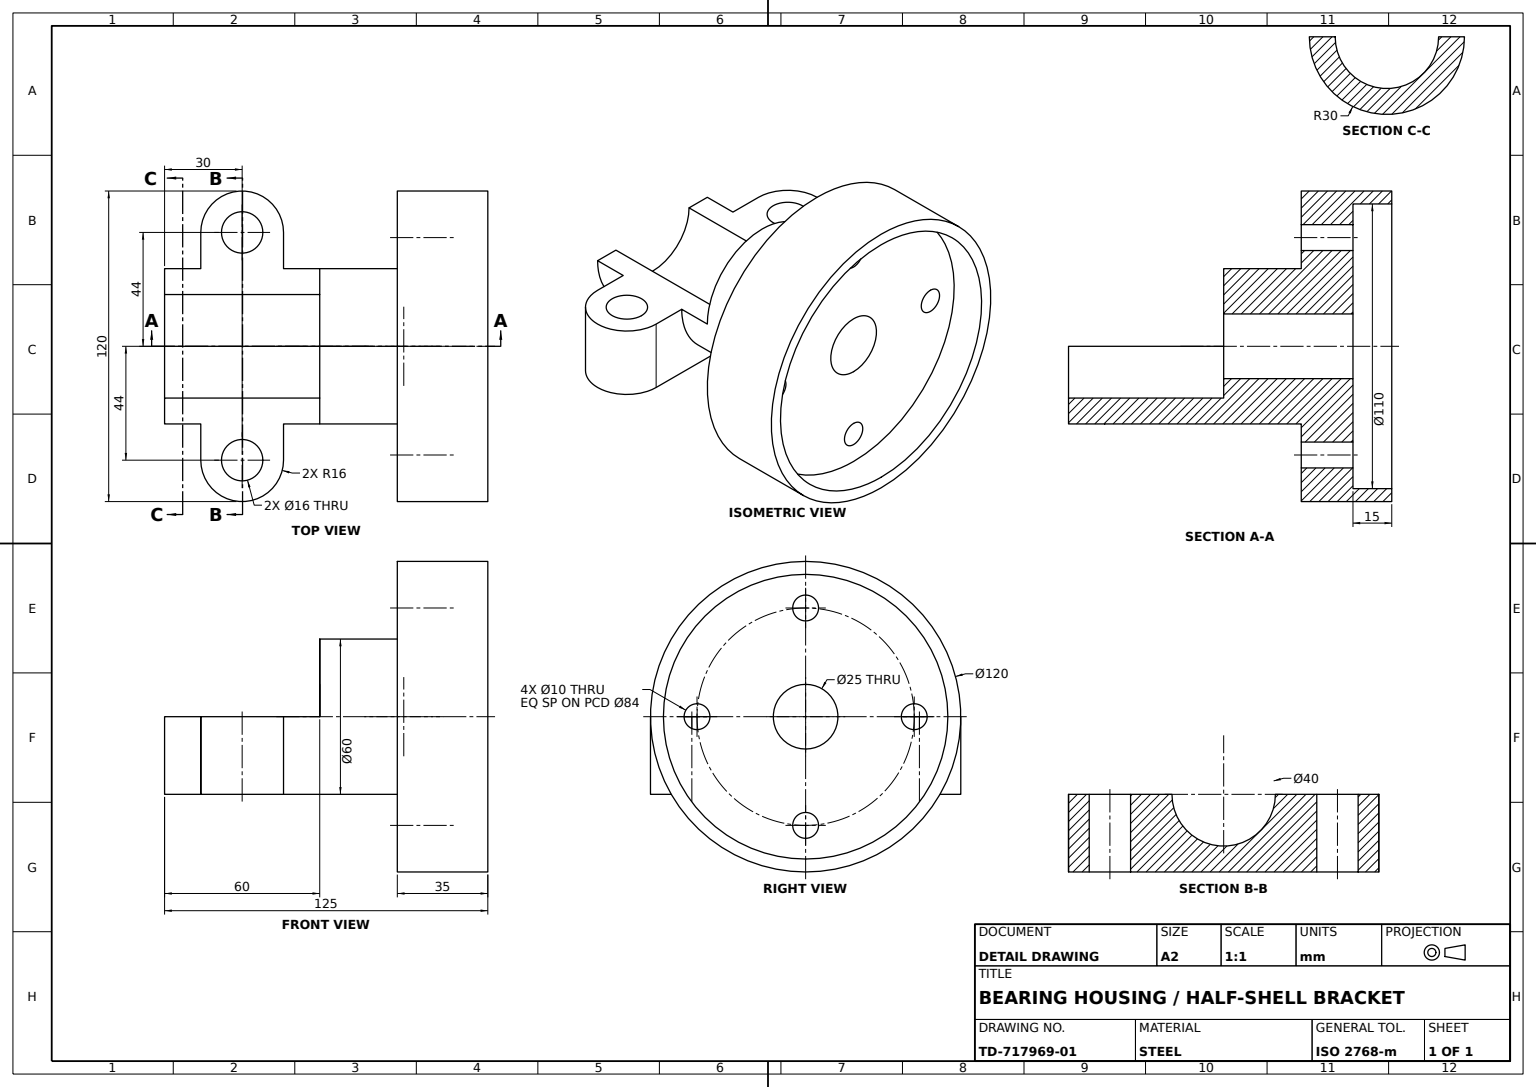
SolidWorks part; units mm, degrees
material "Plain Carbon Steel"
ref_plane "Front Plane" through (0, 0, 0) normal (0, 0, 1) x (1, 0, 0)
ref_plane "Top Plane" through (0, 0, 0) normal (0, 1, 0) x (1, 0, 0)
ref_plane "Right Plane" through (0, 0, 0) normal (1, 0, 0) x (0, 0, -1)
sketch "Flanged Hub Profile" plane through (0, 0, 0) normal (0, 0, 1) x (1, 0, 0)
  line L0 (0, 0) -> (-15, 0) construction
  line L1 (0, 60) -> (-35, 60)
  line L2 (-35, 60) -> (-35, 30)
  line L4 (-15, 12.5) -> (-15, 55)
  line L5 (-15, 55) -> (0, 55)
  line L6 (0, 55) -> (0, 60)
  line L8 (-65, 30) -> (-35, 30)
  line L10 (-65, 30) -> (-65, 12.5)
  line L11 (-65, 12.5) -> (-15, 12.5)
  dimension "D1" = 60
  dimension "D2" = 55
  dimension "D3" = 15
  dimension "D4" = 35
  dimension "D5" = 30
  dimension "D6" = 12.5
  dimension "D7" = 30
revolve "Flanged Hub" add sketch "Flanged Hub Profile" angle 360 about L0
sketch "Flange Bolt Holes Sketch" plane through (-35, 0, 0) normal (-1, 0, 0) x (0, 0, 1)
  circle A0 centre (0, 0) radius 42 construction
  circle A1 centre (42, 0) radius 5
  circle A2 centre (0, -42) radius 5
  circle A3 centre (-42, 0) radius 5
  circle A4 centre (0, 42) radius 5
  dimension "D1" = 84
  dimension "D2" = 10
  dimension "D3" = 4
extrude "Flange Bolt Holes 4xØ10" cut sketch "Flange Bolt Holes Sketch" against normal up to next
sketch "Bearing Block Sketch" plane through (-65, 0, 0) normal (-1, 0, 0) x (0, 0, 1)
  line L0 (-30, 0) -> (-20, 0)
  line L1 (20, 0) -> (30, 0)
  arc A0 (-30, 0) -> (30, 0) centre (0, 0) ccw
  arc A1 (-20, 0) -> (20, 0) centre (0, 0) ccw
  dimension "D1" = 60
  dimension "D2" = 40
extrude "Bearing Block" add sketch "Bearing Block Sketch" along normal blind 60
sketch "Split Cap Lugs Sketch" plane through (0, 0, 0) normal (0, 1, 0) x (1, 0, 0)
  line L0 (-95, -44) -> (-95, 44) construction
  line L1 (-111, -44) -> (-111, 44)
  line L2 (-79, -44) -> (-79, 44)
  line L4 (-125, 20) -> (-125, 30) construction
  arc A0 (-111, -44) -> (-79, -44) centre (-95, -44) ccw
  arc A1 (-79, 44) -> (-111, 44) centre (-95, 44) ccw
  circle A2 centre (-95, 44) radius 8
  circle A3 centre (-95, -44) radius 8
  point P2 (-95, 0)
  dimension "D1" = 16
  dimension "D4" = 16
  dimension "D5" = 16
  dimension "D2" = 30
  dimension "D3" = 44
extrude "Split Cap Lugs" add sketch "Split Cap Lugs Sketch" against normal blind 30
sketch "Journal Seat Split Sketch" plane through (-111, 0, 0) normal (-1, 0, 0) x (0, 0, 1)
  line L1 (20, 0) -> (-20, 0)
  line L2 (20, 0) -> (-20, 0)
  arc A1 (-20, 0) -> (20, 0) centre (0, 0) ccw
  arc A2 (-20, 0) -> (20, 0) centre (0, 0) ccw
  dimension "D1" = 0
extrude "Journal Seat Split Cut" cut sketch "Journal Seat Split Sketch" against normal up to next
